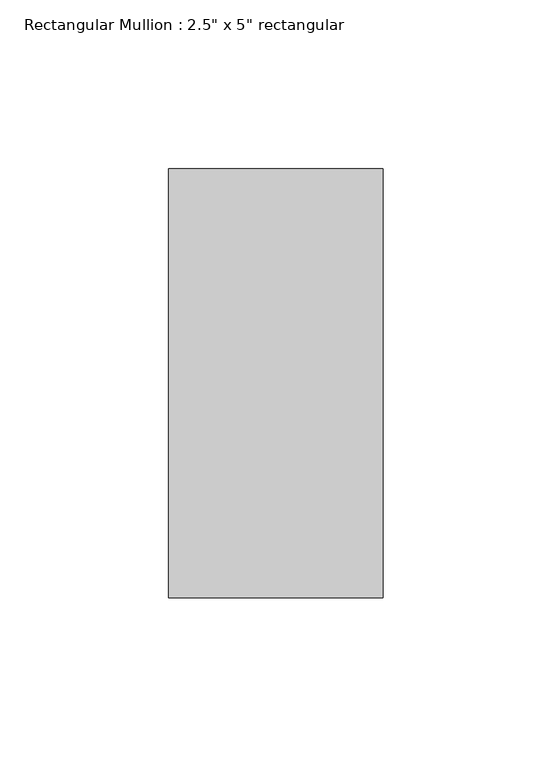
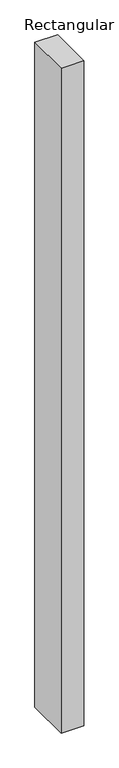
"""IFC4 building model written with IfcOpenShell, lengths in millimetres: member geometry."""

from ifc_helpers import new_model, si_unit, frame, origin, place, context, project, spatial, polyline, outline, extrude, source, transform, mapped, element, save


def member_8a344535(model_context):
    return source(origin(), model_context, "Body", "SweptSolid", [
        extrude(outline(polyline([(0.0, 63.5), (0.0, -63.5), (-63.5, -63.5), (-63.5, 63.5), (0.0, 63.5)])), frame((0.0, 0.0, -1970.8332834), z_axis=(0.0, 0.0, 1.0), x_axis=(1.0, 0.0, 0.0)), (0.0, 0.0, 1.0), 1970.8332834),
    ])


if __name__ == "__main__":
    model = new_model("IFC4")
    model_context = context("Model", 3, world=origin())
    ifc_project = project(units=[si_unit("LENGTHUNIT", "METRE", prefix="MILLI")], contexts=[model_context])
    site = spatial("IfcSite", under=ifc_project)
    building = spatial("IfcBuilding", under=site)
    placement = place(None, origin())
    member_shape = member_8a344535(model_context)
    element("IfcMember", 1, ObjectType="Rectangular Mullion : 2.5\" x 5\" rectangular", at=placement, inside=building, context=model_context, shape_type="MappedRepresentation", body=[
        mapped(member_shape, transform((0.0, 0.0, 0.0), x_axis=(1.0, 0.0, 0.0), y_axis=(0.0, 1.0, 0.0), z_axis=(0.0, 0.0, 1.0))),
    ])
    save(model, "model.ifc")

# Revit data of these elements
# Type "Rectangular Mullion : 2.5\" x 5\" rectangular"
#   built-in parameter 1007304 = 0.416667 (stored number, unit not read)
#   built-in parameter 1007301 = 0.104167 (stored number, unit not read)
#   built-in parameter 1007300 = 0.104167 (stored number, unit not read)
# Element 1 (IfcMember, "Rectangular Mullion : 2.5\" x 5\" rectangular")
#   Materials on its faces: "Aluminum"
# Materials
#   "Aluminum": class "Metal", colour RGB 247 247 247, transparency 0, Description = "Aluminum 6061", Cost = 0
